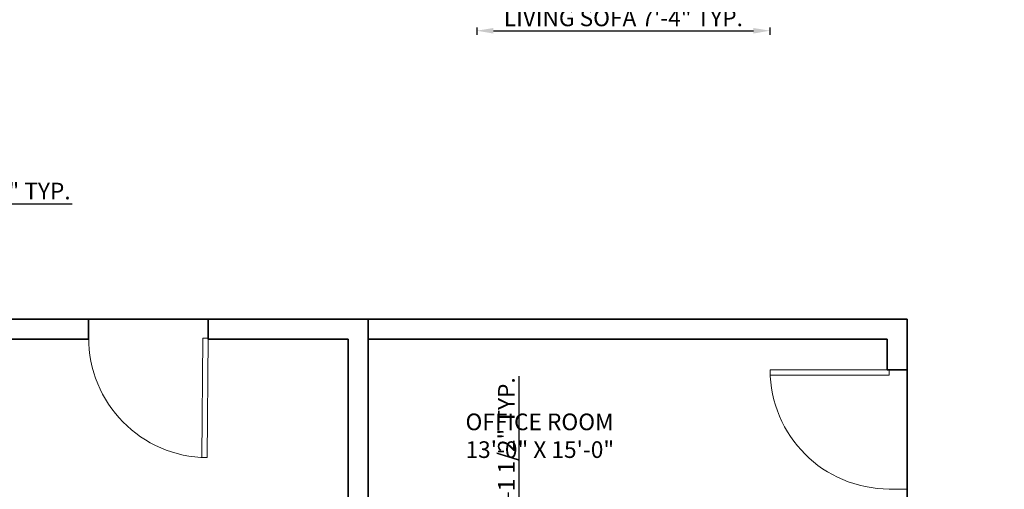
# Model space of a CAD drawing. Units: inches. Extents: x -100 to 766, y -562 to 63.
# Tile 7 of 11: x 152 to 448, y -323 to -182. Entities that reach past the tile are written whole.
import ezdxf

# ---------------------------------------------------------------- set-up
doc = ezdxf.new("R2010")
doc.units = ezdxf.units.IN
for name, color, linetype, lineweight in [('A-ANNO-DIMS', 2, 'Continuous', 18), ('A-AREA-IDEN', 7, 'Continuous', 18), ('A-DOOR', 3, 'Continuous', 18), ('A-WALL', 7, 'Continuous', 35)]:
    doc.layers.add(name, color=color, linetype=linetype, lineweight=lineweight)
doc.styles.get("Standard").update_dxf_attribs({"font": 'arial.ttf'})
doc.dimstyles.new('ISO-25', dxfattribs={"dimtxt": 5, "dimasz": 5, "dimexe": 1.25, "dimexo": 0.625, "dimtad": 1, "dimlunit": 3, "dimtxsty": 'Standard', "dimcen": 2.5, "dimadec": 0, "dimazin": 0, "dimtfac": 1, "dimtmove": 0, "dimatfit": 3, "dimfxl": 1, "dimfxlon": 1, "dimarcsym": 0})

# ---------------------------------------------------------------- blocks, each defined once
blk = doc.blocks.new('*U2')
for p, q in [((0, 0), (0, -6)), ((40, 0), (40, -6))]:
    blk.add_line(p, q)
blk.add_lwpolyline([(0, 0), (0, 40), (1.75, 40), (1.75, 0)], close=True)
blk.add_arc((0, 0), 40, 0, 90)
blk = doc.blocks.new('*D26')
at = {"layer": 'A-ANNO-DIMS', "color": 0, "lineweight": -2, "transparency": 16777216}
for p, q in [((289.04, -184.53), (289.04, -186.78)), ((294.04, -185.53), (372.19, -185.53)), ((377.19, -184.53), (377.19, -186.78))]:
    blk.add_line(p, q, dxfattribs=at)
at = {"layer": 'A-ANNO-DIMS', "color": 0, "transparency": 16777216}
for points in [[(294.04, -184.7), (294.04, -186.37), (289.04, -185.53)], [(372.19, -184.7), (372.19, -186.37), (377.19, -185.53)]]:
    blk.add_solid(points, dxfattribs=at)
at = {"layer": 'Defpoints', "color": 0, "transparency": 16777216}
for p in [(289.04, -172.31), (377.19, -172.31), (377.19, -185.53)]:
    blk.add_point(p, dxfattribs=at)
at = {"layer": 'A-ANNO-DIMS', "color": 0, "transparency": 16777216, "insert": (333.12, -182.32), "char_height": 5, "attachment_point": 5}
blk.add_mtext('LIVING SOFA 7\'-4" TYP.', dxfattribs=at)
blk = doc.blocks.new('*D29')
at = {"layer": 'A-ANNO-DIMS', "color": 0, "lineweight": -2, "transparency": 16777216}
for p, q in [((105.31, -238.5), (105.31, -236.25)), ((127.26, -238.5), (127.26, -236.25)), ((110.31, -237.5), (122.26, -237.5)), ((127.26, -237.5), (167.4, -237.5))]:
    blk.add_line(p, q, dxfattribs=at)
at = {"layer": 'A-ANNO-DIMS', "color": 0, "transparency": 16777216}
for points in [[(110.31, -236.67), (110.31, -238.34), (105.31, -237.5)], [(122.26, -236.67), (122.26, -238.34), (127.26, -237.5)]]:
    blk.add_solid(points, dxfattribs=at)
at = {"layer": 'Defpoints', "color": 0, "transparency": 16777216}
for p in [(127.26, -237.5), (105.31, -241.2), (127.26, -241.2)]:
    blk.add_point(p, dxfattribs=at)
at = {"layer": 'A-ANNO-DIMS', "color": 0, "transparency": 16777216, "insert": (149.83, -234.33), "char_height": 5, "attachment_point": 5}
blk.add_mtext('1\'-10" TYP.', dxfattribs=at)
blk = doc.blocks.new('*D32')
at = {"layer": 'A-ANNO-DIMS', "color": 0, "lineweight": -2, "transparency": 16777216}
for p, q in [((304.17, -335.87), (304.17, -333.62)), ((319.93, -335.87), (319.93, -333.62)), ((309.17, -334.87), (314.93, -334.87)), ((319.93, -334.87), (400.64, -334.87))]:
    blk.add_line(p, q, dxfattribs=at)
at = {"layer": 'A-ANNO-DIMS', "color": 0, "transparency": 16777216}
for points in [[(309.17, -334.04), (309.17, -335.71), (304.17, -334.87)], [(314.93, -334.04), (314.93, -335.71), (319.93, -334.87)]]:
    blk.add_solid(points, dxfattribs=at)
at = {"layer": 'Defpoints', "color": 0, "transparency": 16777216}
for p in [(304.17, -337.24), (319.93, -334.87), (319.93, -337.24)]:
    blk.add_point(p, dxfattribs=at)
at = {"layer": 'A-ANNO-DIMS', "color": 0, "transparency": 16777216, "insert": (362.79, -331.66), "char_height": 5, "attachment_point": 5}
blk.add_mtext('TASK CHAIR 1\'-4" TYP.', dxfattribs=at)
blk = doc.blocks.new('*D33')
at = {"layer": 'A-ANNO-DIMS', "color": 0, "lineweight": -2, "transparency": 16777216}
for p, q in [((301.81, -337.24), (301.81, -289.33)), ((302.81, -337.24), (300.56, -337.24)), ((301.81, -345.65), (301.81, -342.24)), ((302.81, -350.65), (300.56, -350.65))]:
    blk.add_line(p, q, dxfattribs=at)
at = {"layer": 'A-ANNO-DIMS', "color": 0, "transparency": 16777216}
for points in [[(300.98, -342.24), (302.64, -342.24), (301.81, -337.24)], [(300.98, -345.65), (302.64, -345.65), (301.81, -350.65)]]:
    blk.add_solid(points, dxfattribs=at)
at = {"layer": 'Defpoints', "color": 0, "transparency": 16777216}
for p in [(301.81, -337.24), (304.17, -337.24), (304.17, -350.65)]:
    blk.add_point(p, dxfattribs=at)
at = {"layer": 'A-ANNO-DIMS', "color": 0, "transparency": 16777216, "insert": (298.6, -310.78), "char_height": 5, "attachment_point": 5, "rotation": 90}
blk.add_mtext('1\'-1 1/2" TYP.', dxfattribs=at)
blk = doc.blocks.new('*D40')
at = {"layer": 'A-ANNO-DIMS', "color": 0, "lineweight": -2, "transparency": 16777216}
for p, q in [((142.39, -557.16), (142.39, -559.41)), ((147.39, -558.16), (209.39, -558.16)), ((214.39, -557.16), (214.39, -559.41))]:
    blk.add_line(p, q, dxfattribs=at)
at = {"layer": 'A-ANNO-DIMS', "color": 0, "transparency": 16777216}
for points in [[(147.39, -557.32), (147.39, -558.99), (142.39, -558.16)], [(209.39, -557.32), (209.39, -558.99), (214.39, -558.16)]]:
    blk.add_solid(points, dxfattribs=at)
at = {"layer": 'Defpoints', "color": 0, "transparency": 16777216}
for p in [(142.39, -56.21), (214.39, -56.21), (214.39, -558.16)]:
    blk.add_point(p, dxfattribs=at)
at = {"layer": 'A-ANNO-DIMS', "color": 0, "transparency": 16777216, "insert": (178.39, -554.98), "char_height": 5, "attachment_point": 5}
blk.add_mtext('6\'-0"', dxfattribs=at)
blk = doc.blocks.new('*D46')
at = {"layer": 'A-ANNO-DIMS', "color": 0, "lineweight": -2, "transparency": 16777216}
for p, q in [((209.39, -558.16), (204.39, -558.16)), ((214.39, -557.16), (214.39, -559.41)), ((214.39, -558.16), (220.39, -558.16)), ((220.39, -557.16), (220.39, -559.41)), ((225.39, -558.16), (244.93, -558.16))]:
    blk.add_line(p, q, dxfattribs=at)
at = {"layer": 'A-ANNO-DIMS', "color": 0, "transparency": 16777216}
for points in [[(209.39, -557.32), (209.39, -558.99), (214.39, -558.16)], [(225.39, -557.32), (225.39, -558.99), (220.39, -558.16)]]:
    blk.add_solid(points, dxfattribs=at)
at = {"layer": 'Defpoints', "color": 0, "transparency": 16777216}
for p in [(214.39, -182.21), (220.39, -182.21), (220.39, -558.16)]:
    blk.add_point(p, dxfattribs=at)
at = {"layer": 'A-ANNO-DIMS', "color": 0, "transparency": 16777216, "insert": (237.66, -554.98), "char_height": 5, "attachment_point": 5}
blk.add_mtext('0\'-6"', dxfattribs=at)
blk = doc.blocks.new('*D47')
at = {"layer": 'A-ANNO-DIMS', "color": 0, "lineweight": -2, "transparency": 16777216}
for p, q in [((172.42, -557.16), (172.42, -559.41)), ((177.42, -558.16), (203.43, -558.16)), ((208.43, -557.16), (208.43, -559.41))]:
    blk.add_line(p, q, dxfattribs=at)
at = {"layer": 'A-ANNO-DIMS', "color": 0, "transparency": 16777216}
for points in [[(177.42, -557.32), (177.42, -558.99), (172.42, -558.16)], [(203.43, -557.32), (203.43, -558.99), (208.43, -558.16)]]:
    blk.add_solid(points, dxfattribs=at)
at = {"layer": 'Defpoints', "color": 0, "transparency": 16777216}
for p in [(172.42, -182.21), (208.43, -182.21), (208.43, -558.16)]:
    blk.add_point(p, dxfattribs=at)
at = {"layer": 'A-ANNO-DIMS', "color": 0, "transparency": 16777216, "insert": (190.43, -554.98), "char_height": 5, "attachment_point": 5}
blk.add_mtext('3\'-0"', dxfattribs=at)
blk = doc.blocks.new('*D48')
at = {"layer": 'A-ANNO-DIMS', "color": 0, "lineweight": -2, "transparency": 16777216}
for p, q in [((-88.51, -227.21), (-90.76, -227.21)), ((-89.51, -232.21), (-89.51, -252.21)), ((-88.51, -257.21), (-90.76, -257.21))]:
    blk.add_line(p, q, dxfattribs=at)
at = {"layer": 'A-ANNO-DIMS', "color": 0, "transparency": 16777216}
for points in [[(-90.35, -232.21), (-88.68, -232.21), (-89.51, -227.21)], [(-90.35, -252.21), (-88.68, -252.21), (-89.51, -257.21)]]:
    blk.add_solid(points, dxfattribs=at)
at = {"layer": 'Defpoints', "color": 0, "transparency": 16777216}
for p in [(562.39, -227.21), (-89.51, -257.21), (562.39, -257.21)]:
    blk.add_point(p, dxfattribs=at)
at = {"layer": 'A-ANNO-DIMS', "color": 0, "transparency": 16777216, "insert": (-92.69, -242.21), "char_height": 5, "attachment_point": 5, "rotation": 90}
blk.add_mtext('2\'-6"', dxfattribs=at)
blk = doc.blocks.new('*D51')
at = {"layer": 'A-ANNO-DIMS', "color": 0, "lineweight": -2, "transparency": 16777216}
for p, q in [((-88.51, -308.21), (-90.76, -308.21)), ((-89.51, -313.21), (-89.51, -339.21)), ((-88.51, -344.21), (-90.76, -344.21))]:
    blk.add_line(p, q, dxfattribs=at)
at = {"layer": 'A-ANNO-DIMS', "color": 0, "transparency": 16777216}
for points in [[(-90.35, -313.21), (-88.68, -313.21), (-89.51, -308.21)], [(-90.35, -339.21), (-88.68, -339.21), (-89.51, -344.21)]]:
    blk.add_solid(points, dxfattribs=at)
at = {"layer": 'Defpoints', "color": 0, "transparency": 16777216}
for p in [(598.6, -308.21), (-89.51, -344.21), (598.6, -344.21)]:
    blk.add_point(p, dxfattribs=at)
at = {"layer": 'A-ANNO-DIMS', "color": 0, "transparency": 16777216, "insert": (-92.69, -326.21), "char_height": 5, "attachment_point": 5, "rotation": 90}
blk.add_mtext('3\'-0"', dxfattribs=at)
blk = doc.blocks.new('*D56')
at = {"layer": 'A-ANNO-DIMS', "color": 0, "lineweight": -2, "transparency": 16777216}
for p, q in [((220.39, -557.16), (220.39, -559.41)), ((225.39, -558.16), (246.11, -558.16)), ((251.11, -557.16), (251.11, -559.41))]:
    blk.add_line(p, q, dxfattribs=at)
at = {"layer": 'A-ANNO-DIMS', "color": 0, "transparency": 16777216}
for points in [[(225.39, -557.32), (225.39, -558.99), (220.39, -558.16)], [(246.11, -557.32), (246.11, -558.99), (251.11, -558.16)]]:
    blk.add_solid(points, dxfattribs=at)
at = {"layer": 'Defpoints', "color": 0, "transparency": 16777216}
for p in [(220.39, -159.2), (251.11, -159.2), (251.11, -558.16)]:
    blk.add_point(p, dxfattribs=at)
at = {"layer": 'A-ANNO-DIMS', "color": 0, "transparency": 16777216, "insert": (235.75, -554.95), "char_height": 5, "attachment_point": 5}
blk.add_mtext('2\'-6 1/2"', dxfattribs=at)
blk = doc.blocks.new('*D76')
at = {"layer": 'A-ANNO-DIMS', "color": 0, "lineweight": -2, "transparency": 16777216}
for p, q in [((760.28, -228.95), (762.53, -228.95)), ((761.28, -233.95), (761.28, -244.95)), ((760.28, -249.95), (762.53, -249.95))]:
    blk.add_line(p, q, dxfattribs=at)
at = {"layer": 'A-ANNO-DIMS', "color": 0, "transparency": 16777216}
for points in [[(760.45, -233.95), (762.11, -233.95), (761.28, -228.95)], [(760.45, -244.95), (762.11, -244.95), (761.28, -249.95)]]:
    blk.add_solid(points, dxfattribs=at)
at = {"layer": 'Defpoints', "color": 0, "transparency": 16777216}
for p in [(10.38, -228.95), (10.38, -249.95), (761.28, -249.95)]:
    blk.add_point(p, dxfattribs=at)
at = {"layer": 'A-ANNO-DIMS', "color": 0, "transparency": 16777216, "insert": (758.1, -239.45), "char_height": 5, "attachment_point": 5, "rotation": 90}
blk.add_mtext('1\'-9"', dxfattribs=at)
blk = doc.blocks.new('*D78')
at = {"layer": 'A-ANNO-DIMS', "color": 0, "lineweight": -2, "transparency": 16777216}
for p, q in [((208.34, -557.16), (208.34, -559.41)), ((213.34, -558.16), (245.39, -558.16)), ((250.39, -557.16), (250.39, -559.41))]:
    blk.add_line(p, q, dxfattribs=at)
at = {"layer": 'A-ANNO-DIMS', "color": 0, "transparency": 16777216}
for points in [[(213.34, -557.32), (213.34, -558.99), (208.34, -558.16)], [(245.39, -557.32), (245.39, -558.99), (250.39, -558.16)]]:
    blk.add_solid(points, dxfattribs=at)
at = {"layer": 'Defpoints', "color": 0, "transparency": 16777216}
for p in [(208.34, -278.21), (250.39, -278.21), (250.39, -558.16)]:
    blk.add_point(p, dxfattribs=at)
at = {"layer": 'A-ANNO-DIMS', "color": 0, "transparency": 16777216, "insert": (229.37, -554.98), "char_height": 5, "attachment_point": 5}
blk.add_mtext('3\'-6"', dxfattribs=at)
blk = doc.blocks.new('*D79')
at = {"layer": 'A-ANNO-DIMS', "color": 0, "lineweight": -2, "transparency": 16777216}
for p, q in [((216.52, 51.68), (216.52, 53.93)), ((246.52, 51.68), (246.52, 53.93)), ((221.52, 52.68), (241.52, 52.68))]:
    blk.add_line(p, q, dxfattribs=at)
at = {"layer": 'A-ANNO-DIMS', "color": 0, "transparency": 16777216}
for points in [[(221.52, 53.51), (221.52, 51.84), (216.52, 52.68)], [(241.52, 53.51), (241.52, 51.84), (246.52, 52.68)]]:
    blk.add_solid(points, dxfattribs=at)
at = {"layer": 'Defpoints', "color": 0, "transparency": 16777216}
for p in [(246.52, 52.68), (216.52, -362.21), (246.52, -362.21)]:
    blk.add_point(p, dxfattribs=at)
at = {"layer": 'A-ANNO-DIMS', "color": 0, "transparency": 16777216, "insert": (231.52, 55.86), "char_height": 5, "attachment_point": 5}
blk.add_mtext('2\'-6"', dxfattribs=at)
blk = doc.blocks.new('*D81')
at = {"layer": 'A-ANNO-DIMS', "color": 0, "lineweight": -2, "transparency": 16777216}
for p, q in [((-89.51, -273.21), (-89.51, -268.21)), ((-88.51, -278.21), (-90.76, -278.21)), ((-89.51, -278.21), (-89.51, -287.38)), ((-88.51, -287.38), (-90.76, -287.38)), ((-89.51, -292.38), (-89.51, -311.92))]:
    blk.add_line(p, q, dxfattribs=at)
at = {"layer": 'A-ANNO-DIMS', "color": 0, "transparency": 16777216}
for points in [[(-90.35, -273.21), (-88.68, -273.21), (-89.51, -278.21)], [(-90.35, -292.38), (-88.68, -292.38), (-89.51, -287.38)]]:
    blk.add_solid(points, dxfattribs=at)
at = {"layer": 'Defpoints', "color": 0, "transparency": 16777216}
for p in [(412.39, -278.21), (-89.51, -287.38), (412.39, -287.38)]:
    blk.add_point(p, dxfattribs=at)
at = {"layer": 'A-ANNO-DIMS', "color": 0, "transparency": 16777216, "insert": (-92.69, -304.65), "char_height": 5, "attachment_point": 5, "rotation": 90}
blk.add_mtext('0\'-9"', dxfattribs=at)
blk = doc.blocks.new('*D82')
at = {"layer": 'A-ANNO-DIMS', "color": 0, "lineweight": -2, "transparency": 16777216}
for p, q in [((-88.51, -182.21), (-90.76, -182.21)), ((-89.51, -187.21), (-89.51, -222.21)), ((-88.51, -227.21), (-90.76, -227.21))]:
    blk.add_line(p, q, dxfattribs=at)
at = {"layer": 'A-ANNO-DIMS', "color": 0, "transparency": 16777216}
for points in [[(-90.35, -187.21), (-88.68, -187.21), (-89.51, -182.21)], [(-90.35, -222.21), (-88.68, -222.21), (-89.51, -227.21)]]:
    blk.add_solid(points, dxfattribs=at)
at = {"layer": 'Defpoints', "color": 0, "transparency": 16777216}
for p in [(562.39, -182.21), (-89.51, -227.21), (562.39, -227.21)]:
    blk.add_point(p, dxfattribs=at)
at = {"layer": 'A-ANNO-DIMS', "color": 0, "transparency": 16777216, "insert": (-92.69, -204.71), "char_height": 5, "attachment_point": 5, "rotation": 90}
blk.add_mtext('3\'-9"', dxfattribs=at)
blk = doc.blocks.new('*D85')
at = {"layer": 'A-ANNO-DIMS', "color": 0, "lineweight": -2, "transparency": 16777216}
for p, q in [((761.28, -177.21), (761.28, -172.21)), ((760.28, -182.21), (762.53, -182.21)), ((761.28, -182.21), (761.28, -188.21)), ((760.28, -188.21), (762.53, -188.21)), ((761.28, -193.21), (761.28, -212.76))]:
    blk.add_line(p, q, dxfattribs=at)
at = {"layer": 'A-ANNO-DIMS', "color": 0, "transparency": 16777216}
for points in [[(760.45, -177.21), (762.11, -177.21), (761.28, -182.21)], [(760.45, -193.21), (762.11, -193.21), (761.28, -188.21)]]:
    blk.add_solid(points, dxfattribs=at)
at = {"layer": 'Defpoints', "color": 0, "transparency": 16777216}
for p in [(130.39, -182.21), (130.39, -188.21), (761.28, -188.21)]:
    blk.add_point(p, dxfattribs=at)
at = {"layer": 'A-ANNO-DIMS', "color": 0, "transparency": 16777216, "insert": (758.1, -205.49), "char_height": 5, "attachment_point": 5, "rotation": 90}
blk.add_mtext('0\'-6"', dxfattribs=at)
blk = doc.blocks.new('*D87')
at = {"layer": 'A-ANNO-DIMS', "color": 0, "lineweight": -2, "transparency": 16777216}
for p, q in [((310.41, -557.16), (310.41, -559.41)), ((315.41, -558.16), (352.79, -558.16)), ((357.79, -557.16), (357.79, -559.41))]:
    blk.add_line(p, q, dxfattribs=at)
at = {"layer": 'A-ANNO-DIMS', "color": 0, "transparency": 16777216}
for points in [[(315.41, -557.32), (315.41, -558.99), (310.41, -558.16)], [(352.79, -557.32), (352.79, -558.99), (357.79, -558.16)]]:
    blk.add_solid(points, dxfattribs=at)
at = {"layer": 'Defpoints', "color": 0, "transparency": 16777216}
for p in [(310.41, -121.91), (357.79, -121.91), (357.79, -558.16)]:
    blk.add_point(p, dxfattribs=at)
at = {"layer": 'A-ANNO-DIMS', "color": 0, "transparency": 16777216, "insert": (334.1, -554.94), "char_height": 5, "attachment_point": 5}
blk.add_mtext('3\'-11 1/2"', dxfattribs=at)

msp = doc.modelspace()

# ---------------------------------------------------------------- linework, layer by layer
at = {"layer": 'A-WALL'}
for p, q in [((250.388, -272.214), (10.388, -272.214)), ((172.344, -272.214), (172.344, -278.214)), ((208.344, -272.214), (208.344, -278.214)), ((250.388, -272.214), (256.388, -272.214)), ((256.388, -458.214), (256.388, -272.214)), ((256.388, -272.214), (418.394, -272.214)), ((418.394, -458.214), (418.394, -272.214)), ((172.344, -278.214), (10.388, -278.214)), ((250.388, -278.214), (208.344, -278.214)), ((250.388, -362.214), (250.388, -278.214)), ((256.388, -278.214), (262.388, -278.214)), ((262.388, -278.214), (334.388, -278.214)), ((334.388, -278.214), (412.394, -278.214)), ((412.394, -287.377), (412.394, -278.214)), ((412.394, -287.377), (418.394, -287.377))]:
    msp.add_line(p, q, dxfattribs=at)

# ---------------------------------------------------------------- block references
at = {"layer": 'A-DOOR'}
for p, xscale, yscale, zscale, rotation in [((208.3, -277.89), 0.8971966355573497, 0.8971966355573497, 0.8971966355573497, 179.5326886568227), ((413.027, -287.426), -0.8944853722124451, 0.8944853722124451, 0.8944853722124451, 90)]:
    msp.add_blockref('*U2', p, dxfattribs=dict(at, xscale=xscale, yscale=yscale, zscale=zscale, rotation=rotation))

# ---------------------------------------------------------------- texts
at = {"layer": 'A-AREA-IDEN', "insert": (285.675, -300.537), "char_height": 5, "attachment_point": 1}
msp.add_mtext_dynamic_manual_height_columns('OFFICE ROOM\\P13\'-0" X 15\'-0"', width=73.3083, gutter_width=12.5, heights=[0], dxfattribs=at)

# ---------------------------------------------------------------- dimensions: what is measured, and where the dimension line sits
at = {"layer": 'A-ANNO-DIMS'}
for base, p1, p2, picture, middle in [((246.522, 52.678), (216.522, -362.214), (246.522, -362.214), '*D79', (231.522, 55.855)), ((214.388, -558.156), (142.388, -56.214), (214.388, -56.214), '*D40', (178.388, -554.979)), ((357.792, -558.156), (310.414, -121.911), (357.792, -121.911), '*D87', (334.103, -554.944)), ((251.108, -558.156), (220.388, -159.197), (251.108, -159.197), '*D56', (235.748, -554.946)), ((208.434, -558.156), (172.417, -182.214), (208.434, -182.214), '*D47', (190.425, -554.977)), ((220.388, -558.156), (214.388, -182.214), (220.388, -182.214), '*D46', (237.658, -554.979)), ((250.388, -558.156), (208.344, -278.214), (250.388, -278.214), '*D78', (229.366, -554.977))]:
    dim = msp.add_linear_dim(base=base, p1=p1, p2=p2, dimstyle='ISO-25', override={"dimdec": 1, "dimlfac": 1, "dimrnd": 0, "dimzin": 1, "dimdsep": 46, "dimlunit": 4, "dimfrac": 2}, dxfattribs=at)
    dim.commit()
    dim.dimension.update_dxf_attribs({"geometry": picture, "text_midpoint": middle})
for base, p1, p2, text, picture, middle in [((377.186, -185.532), (289.045, -172.311), (377.186, -172.311), 'LIVING SOFA <> TYP.', '*D26', (333.115, -182.32)), ((127.257, -237.504), (105.312, -241.202), (127.257, -241.202), '<> TYP.', '*D29', (149.828, -234.327)), ((319.931, -334.874), (304.173, -337.238), (319.931, -337.238), 'TASK CHAIR <> TYP.', '*D32', (362.787, -331.664))]:
    dim = msp.add_linear_dim(base=base, p1=p1, p2=p2, text=text, dimstyle='ISO-25', override={"dimdec": 1, "dimlfac": 1, "dimrnd": 0, "dimzin": 1, "dimdsep": 46, "dimlunit": 4, "dimfrac": 2}, dxfattribs=at)
    dim.commit()
    dim.dimension.update_dxf_attribs({"geometry": picture, "text_midpoint": middle})
for base, p1, p2, picture, middle in [((761.28, -188.214), (130.388, -182.214), (130.388, -188.214), '*D85', (758.102, -205.485)), ((-89.513, -227.214), (562.394, -182.214), (562.394, -227.214), '*D82', (-92.693, -204.714)), ((-89.513, -257.214), (562.394, -227.214), (562.394, -257.214), '*D48', (-92.691, -242.214)), ((761.28, -249.949), (10.379, -228.949), (10.379, -249.949), '*D76', (758.102, -239.449)), ((-89.513, -287.377), (412.394, -278.214), (412.394, -287.377), '*D81', (-92.691, -304.648)), ((-89.513, -344.214), (598.603, -308.214), (598.603, -344.214), '*D51', (-92.693, -326.214))]:
    dim = msp.add_linear_dim(base=base, p1=p1, p2=p2, angle=90, dimstyle='ISO-25', override={"dimdec": 1, "dimlfac": 1, "dimrnd": 0, "dimzin": 1, "dimdsep": 46, "dimlunit": 4, "dimfrac": 2}, dxfattribs=at)
    dim.commit()
    dim.dimension.update_dxf_attribs({"geometry": picture, "text_midpoint": middle})
dim = msp.add_linear_dim(base=(301.81, -337.238), p1=(304.173, -350.654), p2=(304.173, -337.238), angle=90, text='<> TYP.', dimstyle='ISO-25', override={"dimdec": 1, "dimlfac": 1, "dimrnd": 0, "dimzin": 1, "dimdsep": 46, "dimlunit": 4, "dimfrac": 2}, dxfattribs=at)
dim.commit()
dim.dimension.update_dxf_attribs({"geometry": '*D33', "text_midpoint": (298.6, -310.784)})

doc.saveas('drawing.dxf')
